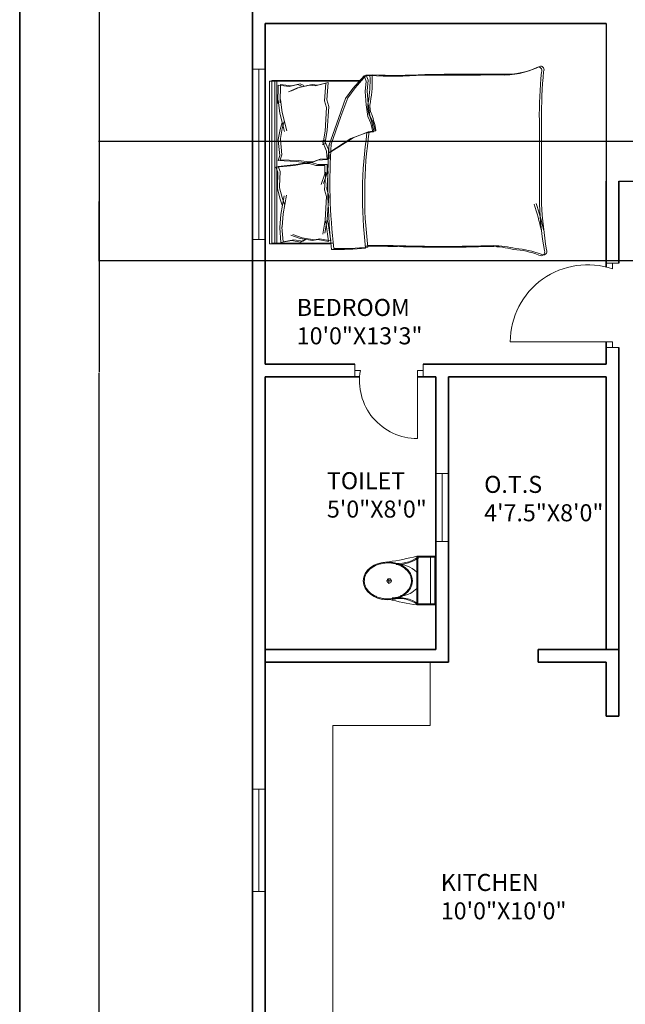
# Model space of a CAD drawing. Units: inches. Extents: x 1088 to 1703, y 668 to 1875.
# Tile 2 of 45: x 1088 to 1302, y 1069 to 1416. Entities that reach past the tile are written whole.
import ezdxf

# ---------------------------------------------------------------- set-up
doc = ezdxf.new("R2010")
doc.units = ezdxf.units.IN
for name, color, linetype, lineweight in [('A-ANNO-DIMS', 2, 'Continuous', 18), ('A-ANNO-TTLB', 7, 'Continuous', 35), ('A-AREA-IDEN', 7, 'Continuous', 18), ('A-DOOR', 4, 'Continuous', 18), ('A-FLOR-CASE', 8, 'Continuous', 18), ('A-FLOR-EVTR', 5, 'Continuous', 25), ('A-FLOR-FIXT', 8, 'Continuous', 18), ('A-FURN', 8, 'Continuous', 13), ('A-GLAZ', 4, 'Continuous', 18), ('A-WALL', 7, 'Continuous', 35)]:
    doc.layers.add(name, color=color, linetype=linetype, lineweight=lineweight)
doc.styles.get("Standard").update_dxf_attribs({"font": 'arial.ttf'})
doc.dimstyles.get("Standard").update_dxf_attribs({"dimtxt": 0.18, "dimasz": 0.18, "dimexe": 0.18, "dimexo": 0.0625, "dimgap": 0.09, "dimtad": 0, "dimtih": 1, "dimtoh": 1, "dimdec": 4, "dimzin": 0, "dimdsep": 46, "dimtxsty": 'Standard', "dimcen": 0.09, "dimadec": 0, "dimazin": 0, "dimtfac": 1, "dimtdec": 4, "dimtofl": 0, "dimtmove": 0, "dimatfit": 3, "dimfxl": 1, "dimtolj": 1, "dimtzin": 0, "dimarcsym": 0})

# ---------------------------------------------------------------- blocks, each defined once
blk = doc.blocks.new('A$C31115884')
for p, q in [((283, 498), (223, 498)), ((258, 466), (258, 523)), ((0, 200), (0, 0)), ((520, 200), (0, 200)), ((10, 190), (10, 10)), ((510, 190), (10, 190)), ((510, 10), (510, 190)), ((520, 0), (520, 200)), ((510, 54), (0, 54)), ((10, 10), (510, 10)), ((0, 0), (520, 0))]:
    blk.add_line(p, q)
blk.add_circle((256, 496), 23.6)
for centre, radius, start, end in [((2778, -205), 2807, 165.4549, 171.7133), ((-295, 403), 365, 324.2091, 9.3499), ((-295, 403), 375, 324.2091, 9.3499), ((139, 406), 293, 315.8436, 2.6563), ((806, 403), 365, 170.6501, 215.7909), ((3237, 905), 2807, 188.2867, 194.5451), ((384, 406), 293, 190.2774, 224.1564), ((806, 403), 375, 179.2036, 215.7909)]:
    blk.add_arc(centre, radius, start, end)
blk.add_ellipse((256, 510), major_axis=(0, -261), ratio=0.772727)
blk.add_open_spline([(256, 259), (263, 259), (270, 260), (288, 262), (299, 265), (320, 273), (330, 278), (350, 291), (360, 299), (378, 316), (386, 326), (402, 347), (409, 358), (421, 383), (427, 395), (436, 422), (440, 436), (445, 465), (447, 480), (448, 509), (448, 524), (445, 553), (443, 568), (436, 596), (432, 610), (422, 636), (416, 649), (402, 672), (395, 683), (379, 703), (370, 712), (351, 728), (341, 735), (321, 746), (310, 751), (289, 757), (278, 759), (256, 761), (245, 761), (223, 757), (212, 754), (191, 746), (181, 741), (161, 728), (151, 720), (133, 703), (125, 693), (110, 672), (103, 660), (90, 636), (85, 623), (76, 596), (72, 582), (67, 553), (66, 538), (64, 509), (65, 494), (68, 465), (70, 450), (77, 422), (81, 408), (91, 382), (97, 370), (111, 346), (118, 335), (135, 316), (144, 307), (162, 291), (172, 284), (193, 273), (203, 269), (225, 262), (236, 260), (250, 259), (253, 259), (256, 259)], degree=3, knots=[0, 0, 0, 0, 0.110105, 0.110105, 0.285049, 0.285049, 0.459994, 0.459994, 0.634938, 0.634938, 0.809882, 0.809882, 0.984827, 0.984827, 1.159771, 1.159771, 1.334715, 1.334715, 1.50966, 1.50966, 1.684604, 1.684604, 1.859549, 1.859549, 2.034493, 2.034493, 2.209437, 2.209437, 2.384382, 2.384382, 2.559326, 2.559326, 2.73427, 2.73427, 2.909215, 2.909215, 3.084159, 3.084159, 3.259103, 3.259103, 3.434048, 3.434048, 3.608992, 3.608992, 3.783936, 3.783936, 3.958881, 3.958881, 4.133825, 4.133825, 4.30877, 4.30877, 4.483714, 4.483714, 4.658658, 4.658658, 4.833603, 4.833603, 5.008547, 5.008547, 5.183491, 5.183491, 5.358436, 5.358436, 5.53338, 5.53338, 5.708324, 5.708324, 5.883269, 5.883269, 6.058213, 6.058213, 6.233158, 6.233158, 6.283185, 6.283185, 6.283185, 6.283185])
blk = doc.blocks.new('BED-DOUBLE')
for p, q in [((33.26, 63.38), (29.37, 58.94)), ((34.03, 63.65), (30.13, 59.21)), ((35.35, 63.48), (33.26, 63.38, 4.64)), ((34.01, 61.54), (33.26, 63.38)), ((36.12, 63.75), (34.03, 63.65, 4.64)), ((34.77, 61.81), (34.03, 63.65)), ((0, 61.46), (31.9, 61.46)), ((0, 4.17), (0, 61.46)), ((0.77, 61.73), (32.67, 61.73)), ((0.77, 4.44), (0.77, 61.73)), ((1.84, 4.17), (1.84, 61.46)), ((2.6, 4.44), (2.6, 61.73)), ((3.07, 60.08), (2.95, 53.6)), ((3.07, 60.08), (6.91, 59.62)), ((3.83, 60.35), (3.72, 53.87)), ((3.83, 60.35), (7.68, 59.9)), ((9.9, 59.12), (6.69, 57.7)), ((6.91, 59.62), (10, 60.34)), ((10.67, 59.39), (7.45, 57.97)), ((7.68, 59.9), (10.76, 60.61)), ((14.18, 60.08), (9.9, 59.12)), ((10, 60.34), (11.25, 59.72)), ((14.95, 60.35), (10.67, 59.39)), ((10.76, 60.61), (12.02, 59.99)), ((16.11, 59.85), (14.18, 60.08)), ((16.87, 60.12), (14.95, 60.35)), ((19.87, 60.78), (16.11, 59.85)), ((20.63, 61.05), (16.87, 60.12)), ((19.38, 54.63), (19.87, 60.78)), ((20.15, 54.9), (20.63, 61.05)), ((30.13, 59.21), (27.54, 55.68)), ((33.63, 57.82), (34.01, 61.54)), ((34.4, 58.1), (34.77, 61.81)), ((27.54, 55.68), (25.12, 49)), ((29.37, 58.94), (26.77, 55.41)), ((34.01, 53.18), (33.63, 57.82)), ((34.77, 53.46), (34.4, 58.1)), ((2.95, 53.6), (3.05, 54.8)), ((3.05, 54.8), (3.68, 50.25)), ((3.72, 53.87), (3.81, 55.08)), ((3.81, 55.08), (4.45, 50.52)), ((20.05, 52.28), (19.38, 54.63)), ((19.54, 43.87), (20.05, 52.28)), ((20.82, 52.55), (20.15, 54.9)), ((20.3, 44.15), (20.82, 52.55)), ((26.77, 55.41), (24.36, 48.73)), ((34.56, 49.1), (34.01, 53.18)), ((35.33, 49.37), (34.77, 53.46)), ((3.68, 50.25), (5.3, 43.75)), ((4.45, 50.52), (6.07, 44.03)), ((24.36, 48.73), (20.84, 38.73)), ((25.12, 49), (21.61, 39)), ((35.68, 46.68), (34.56, 49.1)), ((36.44, 46.96), (35.33, 49.37)), ((4.4, 47), (3.69, 44.52)), ((5.17, 47.27), (4.46, 44.79)), ((36.42, 43.71), (35.68, 46.68)), ((37.18, 43.99), (36.44, 46.96)), ((95, 18.06), (95, 47.57)), ((95.77, 18.33), (95.77, 47.84)), ((3.69, 44.52), (3.04, 41.01)), ((4.46, 44.79), (3.81, 41.28)), ((18.74, 39.04), (19.54, 43.87)), ((19.5, 39.31), (20.3, 44.15)), ((28.62, 41.3), (34.01, 43.34)), ((29.39, 41.57), (34.77, 43.62)), ((34.01, 43.34), (36.42, 43.71)), ((34.77, 43.62), (37.18, 43.99)), ((3.04, 41.01), (3.07, 40.62)), ((3.07, 40.62), (3.57, 35.31)), ((3.81, 41.28), (3.83, 40.9)), ((3.83, 40.9), (4.34, 35.59)), ((20.07, 36.87), (18.53, 40.55)), ((20.83, 37.14), (19.29, 40.82)), ((20.84, 36.28), (28.62, 41.3)), ((21.61, 36.55), (29.39, 41.57)), ((3.57, 35.31), (2.99, 33.54)), ((4.34, 35.59), (3.75, 33.81)), ((20.25, 33.93), (20.07, 36.87)), ((21.02, 34.2), (20.83, 37.14)), ((2.24, 31.15), (8.66, 31.84)), ((2.99, 33.54), (9.43, 33.25)), ((3.01, 31.42), (9.42, 32.12)), ((3.7, 29.69), (3.01, 31.42)), ((3.75, 33.81), (10.2, 33.52)), ((8.66, 31.84), (12.47, 32.54)), ((9.42, 32.12), (13.24, 32.81)), ((9.43, 33.25), (13.28, 32.79)), ((10.2, 33.52), (14.05, 33.07)), ((12.47, 32.54), (14.03, 32.54)), ((13.24, 32.81), (14.8, 32.81)), ((13.28, 32.79), (14.84, 32.89)), ((14.03, 32.54), (16.28, 31.84)), ((14.05, 33.07), (15.6, 33.17)), ((14.8, 32.81), (17.05, 32.12)), ((14.84, 32.89), (17.04, 33.72)), ((15.6, 33.17), (17.81, 34)), ((16.28, 31.84), (19.5, 31.84)), ((17.04, 33.72), (20.25, 33.93)), ((17.05, 32.12), (20.26, 32.12)), ((17.81, 34), (21.02, 34.2)), ((19.5, 31.84), (19.5, 28.9)), ((20.26, 32.12), (20.26, 29.17)), ((2.94, 29.42), (2.24, 31.15)), ((2.76, 24.09), (2.94, 29.42)), ((3.53, 24.36), (3.7, 29.69)), ((19.5, 28.9), (18.19, 25.13)), ((20.26, 29.17), (18.96, 25.4)), ((19.38, 23.24), (19.87, 29.39)), ((20.15, 23.51), (20.63, 29.67)), ((3.53, 23.98), (3.53, 24.36)), ((2.76, 23.7), (2.76, 24.09)), ((3.63, 20.24), (2.76, 23.7)), ((4.4, 20.51), (3.53, 23.98)), ((3.98, 14.52), (5.19, 21.1)), ((4.74, 14.79), (5.96, 21.38)), ((20.05, 20.89), (19.38, 23.24)), ((19.54, 12.48), (20.05, 20.89)), ((20.82, 21.16), (20.15, 23.51)), ((20.3, 12.76), (20.82, 21.16)), ((4.5, 17.81), (3.63, 20.24)), ((5.26, 18.08), (4.4, 20.51)), ((3.63, 9.93), (3.98, 14.52)), ((4.4, 10.21), (4.74, 14.79)), ((18.74, 7.65), (19.54, 12.48)), ((19.5, 7.92), (20.3, 12.76)), ((19.54, 12.48), (19.92, 11.13)), ((19.92, 11.13), (20.79, 5.02)), ((20.3, 12.76), (20.69, 11.4)), ((20.69, 11.4), (21.56, 5.29)), ((3.61, 9.81), (3.63, 9.93)), ((4, 4.67), (3.61, 9.81)), ((4.37, 10.08), (4.4, 10.21)), ((4.77, 4.95), (4.37, 10.08)), ((10.74, 6.06), (7.44, 7.27)), ((11.5, 6.33), (8.21, 7.54)), ((21.71, 4.17), (0, 4.17)), ((22.48, 4.44), (0.77, 4.44)), ((3.98, 4.67), (7.79, 5.36)), ((4.74, 4.94), (8.56, 5.64)), ((7.79, 5.36), (10.91, 4.84)), ((8.56, 5.64), (11.68, 5.12)), ((15.07, 5.36), (10.74, 6.06)), ((10.91, 4.84), (12.12, 5.54)), ((15.84, 5.64), (11.5, 6.33)), ((11.68, 5.12), (12.89, 5.81)), ((16.98, 5.71), (15.07, 5.36)), ((17.74, 5.98), (15.84, 5.64)), ((20.79, 5.02), (16.98, 5.71)), ((21.56, 5.29), (17.74, 5.98))]:
    blk.add_line(p, q)
for centre, radius, start, end in [((82.32, 91.3), 27.65, 267.4714, 296.4681), ((83.09, 91.58), 27.65, 267.4714, 296.4681), ((94.55, 65.23), 1.32, 332.6588, 86.02), ((95.32, 65.5), 1.32, 332.6588, 86.02), ((-7.98, 61.53), 43.38, 349.8763, 2.5657), ((43.54, 218.51), 155.25, 266.9791, 273.8365), ((-7.21, 61.81), 43.38, 349.8763, 2.5657), ((44.3, 218.78), 155.25, 266.9791, 273.8365), ((81.31, -5405.34), 5469.02, 90.00217, 90.28689), ((82.07, -5405.07), 5469.02, 90.00217, 90.28689), ((254.49, 49.34), 159.5, 174.4998, 180.6351), ((255.26, 49.61), 159.5, 174.4998, 180.6351), ((42.04, 52.44), 7.46, 168.6608, 203.7384), ((42.81, 52.72), 7.46, 168.6608, 203.7384), ((1.78, 37.35), 35.55, 10.6617, 19.8806), ((2.54, 37.62), 35.55, 10.6617, 19.8806), ((187.4, 21.29), 154.68, 171.7845, 186.9006), ((188.17, 21.56), 154.68, 171.7845, 186.9006), ((36.49, 43.92), 0.221, 250.2464, 1.1377), ((37.26, 44.2), 0.221, 250.2464, 1.1377), ((218.25, 25.61), 197.77, 176.0865, 186.7821), ((219.02, 25.88), 197.77, 176.0865, 186.7821), ((-28.43, -20.65), 127.63, 13.3832, 17.7053), ((-27.66, -20.37), 127.63, 13.3832, 17.7053), ((240.78, 25.69), 145.97, 182.9958, 189.4091), ((241.54, 25.96), 145.97, 182.9958, 189.4091), ((38.14, -200.3), 203.94, 88.4762, 91.0082), ((61.45, 581.51), 578.22, 268.22771, 271.71854), ((78.11, -31.97), 35.53, 76.0648, 88.9113), ((24.09, 102.1), 99.87, 268.7218, 275.604), ((24.86, 102.37), 99.87, 268.7218, 275.604), ((37.37, -200.58), 203.94, 88.4762, 91.0082), ((60.68, 581.23), 578.22, 268.22771, 271.71854), ((77.34, -32.25), 35.53, 76.0648, 88.9113), ((84.25, -25.97), 28.25, 67.9751, 86.652), ((85.02, -25.69), 28.25, 67.9751, 86.652), ((95.57, 1.3), 1.31, 236.1736, 23.4781), ((96.34, 1.58), 1.31, 236.1736, 23.4781)]:
    blk.add_arc(centre, radius, start, end)
blk = doc.blocks.new('WIN-24-RETURN')
for p, q in [((0, 24), (4.5, 24)), ((4.5, 24), (2.25, 24)), ((2.25, 24), (2.25, 0)), ((4.5, 0), (0, 0)), ((2.25, 0), (4.5, 0))]:
    blk.add_line(p, q)
blk = doc.blocks.new('DOOR-SWING-24')
for p, q in [((4.5, 24.09), (0, 24.09)), ((0, 24.09), (2.25, 24.09)), ((2.25, 24.09), (2.25, 22.09)), ((2.25, 22.09), (26.25, 22.09)), ((0, 0), (4.5, 0)), ((2.25, 0), (2.25, 2)), ((4.5, 0), (2.25, 0))]:
    blk.add_line(p, q)
blk.add_arc((5.84, 22.09), 20.41, 259.876, 0)
blk = doc.blocks.new('*D29')
at = {"layer": 'A-ANNO-DIMS', "color": 0, "lineweight": -2, "transparency": 16777216}
for p, q in [((1170.28, 1803.56), (1116.11, 1803.56)), ((1116.29, 1803.38), (1116.29, 1291.85)), ((1116.29, 779.96), (1116.29, 1291.49)), ((1170.28, 779.78), (1116.11, 779.78))]:
    blk.add_line(p, q, dxfattribs=at)
at = {"layer": 'A-ANNO-DIMS', "color": 0, "transparency": 16777216}
for points in [[(1116.26, 1803.38), (1116.32, 1803.38), (1116.29, 1803.56)], [(1116.26, 779.96), (1116.32, 779.96), (1116.29, 779.78)]]:
    blk.add_solid(points, dxfattribs=at)
at = {"layer": 'Defpoints', "color": 0, "transparency": 16777216}
for p in [(1116.29, 1803.56), (1170.34, 1803.56), (1170.34, 779.78)]:
    blk.add_point(p, dxfattribs=at)
at = {"layer": 'A-ANNO-DIMS', "color": 0, "transparency": 16777216, "insert": (1116.29, 1291.67), "char_height": 0.18, "attachment_point": 5}
blk.add_mtext('\\A1;1023.8', dxfattribs=at)
blk = doc.blocks.new('*D34')
at = {"layer": 'A-ANNO-DIMS', "color": 0, "lineweight": -2, "transparency": 16777216}
for p, q in [((1460.53, 1373.06), (1116.11, 1373.06)), ((1116.29, 1372.88), (1116.29, 1352.24)), ((1116.29, 1331.24), (1116.29, 1351.88)), ((1460.53, 1331.06), (1116.11, 1331.06))]:
    blk.add_line(p, q, dxfattribs=at)
at = {"layer": 'A-ANNO-DIMS', "color": 0, "transparency": 16777216}
for points in [[(1116.26, 1372.88), (1116.32, 1372.88), (1116.29, 1373.06)], [(1116.26, 1331.24), (1116.32, 1331.24), (1116.29, 1331.06)]]:
    blk.add_solid(points, dxfattribs=at)
at = {"layer": 'Defpoints', "color": 0, "transparency": 16777216}
for p in [(1116.29, 1373.06), (1460.59, 1373.06), (1460.59, 1331.06)]:
    blk.add_point(p, dxfattribs=at)
at = {"layer": 'A-ANNO-DIMS', "color": 0, "transparency": 16777216, "insert": (1116.29, 1352.06), "char_height": 0.18, "attachment_point": 5}
blk.add_mtext('\\A1;42', dxfattribs=at)

msp = doc.modelspace()

# ---------------------------------------------------------------- linework, layer by layer
at = {"layer": 'A-ANNO-TTLB'}
msp.add_lwpolyline([(1088.369, 1874.677), (1703.181, 1874.677), (1703.181, 667.947), (1088.369, 667.947)], close=True, dxfattribs=at)
at = {"layer": 'A-DOOR'}
for p, q in [((1294.845, 1330.162), (1299.345, 1330.162)), ((1299.345, 1330.162), (1297.095, 1330.162)), ((1297.095, 1330.162), (1297.095, 1328.162)), ((1297.095, 1302.46), (1261.095, 1302.46)), ((1297.095, 1300.46), (1297.095, 1302.46)), ((1299.345, 1300.46), (1294.845, 1300.46)), ((1294.845, 1300.46), (1297.095, 1300.46))]:
    msp.add_line(p, q, dxfattribs=at)
msp.add_arc((1288.27, 1302.46), 27.175, 71.05065, 180, dxfattribs=at)
at = {"layer": 'A-FLOR-CASE'}
for p, q in [((1232.862, 1167.334), (1232.862, 1189.644)), ((1198.631, 1029.558), (1198.631, 1167.334)), ((1198.631, 1167.334), (1232.862, 1167.334))]:
    msp.add_line(p, q, dxfattribs=at)
at = {"layer": 'A-FLOR-EVTR'}
for p, q in [((1294.845, 1414.644), (1294.845, 1359.144)), ((1294.845, 1414.644), (1294.845, 1359.144)), ((1294.845, 1414.644), (1294.845, 1410.144)), ((1299.345, 1359.144), (1350.345, 1359.144))]:
    msp.add_line(p, q, dxfattribs=at)
at = {"layer": 'A-GLAZ'}
for p, q in [((1174.845, 1398.555), (1170.345, 1398.555)), ((1170.345, 1398.555), (1172.595, 1398.555)), ((1172.595, 1398.555), (1172.595, 1338.555)), ((1174.845, 1338.555), (1170.345, 1338.555)), ((1172.595, 1338.555), (1174.845, 1338.555)), ((1174.845, 1144.851), (1170.345, 1144.851)), ((1170.345, 1144.851), (1172.595, 1144.851)), ((1172.595, 1144.851), (1172.595, 1108.851)), ((1174.845, 1108.851), (1170.345, 1108.851)), ((1172.595, 1108.851), (1174.845, 1108.851))]:
    msp.add_line(p, q, dxfattribs=at)
at = {"layer": 'A-WALL'}
for p, q in [((1170.345, 1803.558), (1170.345, 836.058)), ((1174.845, 1414.644), (1294.845, 1414.644)), ((1174.845, 1414.644), (1294.845, 1414.644)), ((1174.845, 1414.644), (1174.845, 1294.644)), ((1174.845, 1414.644), (1174.845, 1325.058)), ((1294.845, 1359.144), (1294.845, 1328.828)), ((1299.345, 1330.162), (1299.345, 1359.144)), ((1294.845, 1302.46), (1294.845, 1294.644)), ((1299.345, 1290.144), (1299.345, 1300.46)), ((1174.845, 1294.644), (1206.313, 1294.644)), ((1230.404, 1294.644), (1294.845, 1294.644)), ((1234.845, 1294.644), (1239.345, 1294.644)), ((1174.845, 1290.144), (1208.039, 1290.144)), ((1174.845, 1290.144), (1174.845, 1194.144)), ((1228.404, 1290.144), (1234.845, 1290.144)), ((1234.845, 1194.144), (1234.845, 1290.144)), ((1239.345, 1290.144), (1239.345, 1194.144)), ((1239.345, 1290.144), (1294.845, 1290.144)), ((1294.845, 1194.144), (1294.845, 1290.144)), ((1299.345, 1290.144), (1299.345, 1189.644)), ((1174.845, 1220.058), (1174.845, 1069.644)), ((1174.845, 1194.144), (1234.845, 1194.144)), ((1174.845, 1194.144), (1234.845, 1194.144)), ((1239.345, 1194.144), (1239.345, 1189.644)), ((1270.961, 1194.144), (1294.845, 1194.144)), ((1270.961, 1194.144), (1270.961, 1189.644)), ((1294.845, 1194.144), (1299.345, 1194.144)), ((1174.845, 1189.644), (1239.345, 1189.644)), ((1174.845, 1189.644), (1174.845, 1069.644)), ((1174.845, 1189.644), (1174.845, 1029.558)), ((1270.961, 1189.644), (1294.845, 1189.644)), ((1270.961, 1189.644), (1294.845, 1189.644)), ((1294.845, 1170.556), (1294.845, 1189.644)), ((1299.345, 1189.644), (1299.345, 1170.556)), ((1299.345, 1170.556), (1294.845, 1170.556))]:
    msp.add_line(p, q, dxfattribs=at)

# ---------------------------------------------------------------- block references
at = {"layer": 'A-DOOR', "rotation": 269.9964663852828}
msp.add_blockref('DOOR-SWING-24', (1206.311, 1294.645), dxfattribs=at)
at = {"layer": 'A-FLOR-FIXT', "xscale": 0.0330640103915726, "yscale": 0.0330640103915726, "zscale": 0.0330640103915726, "rotation": 89.99999999999996}
msp.add_blockref('A$C31115884', (1234.845, 1209.801), dxfattribs=at)
at = {"layer": 'A-FURN'}
msp.add_blockref('BED-DOUBLE', (1176.337, 1332.816), dxfattribs=at)
at = {"layer": 'A-GLAZ'}
msp.add_blockref('WIN-24-RETURN', (1234.845, 1232.13), dxfattribs=at)

# ---------------------------------------------------------------- texts
at = {"layer": 'A-AREA-IDEN', "char_height": 6, "attachment_point": 1}
for s, width, insert in [('BEDROOM\\P10\'0"X13\'3"', 246.13777, (1185.914, 1317.604)), ('TOILET\\P5\'0"X8\'0"', 67.92603, (1196.543, 1256.571)), ('O.T.S\\P4\'7.5"X8\'0"', 74.68718, (1251.902, 1255.27)), ('KITCHEN\\P10\'0"X10\'0"', 104.87486, (1236.639, 1115.028))]:
    msp.add_mtext_dynamic_manual_height_columns(s, width=width, gutter_width=12.5, heights=[0], dxfattribs=dict(at, insert=insert))

# ---------------------------------------------------------------- dimensions: what is measured, and where the dimension line sits
at = {"layer": 'A-ANNO-DIMS'}
for base, p1, p2, override, picture, middle in [((1116.295, 1803.558), (1170.345, 779.779), (1170.345, 1803.558), {"dimdec": 1, "dimlfac": 1, "dimrnd": 0, "dimzin": 0, "dimdsep": 46, "dimlunit": 2}, '*D29', (1116.295, 1291.669)), ((1116.295, 1373.058), (1460.595, 1331.058), (1460.595, 1373.058), {"dimdec": 0, "dimlfac": 1, "dimrnd": 0, "dimzin": 0, "dimdsep": 46, "dimlunit": 2}, '*D34', (1116.295, 1352.058))]:
    dim = msp.add_linear_dim(base=base, p1=p1, p2=p2, angle=90, dimstyle='Standard', override=override, dxfattribs=at)
    dim.commit()
    dim.dimension.update_dxf_attribs({"geometry": picture, "text_midpoint": middle})

doc.saveas('drawing.dxf')
